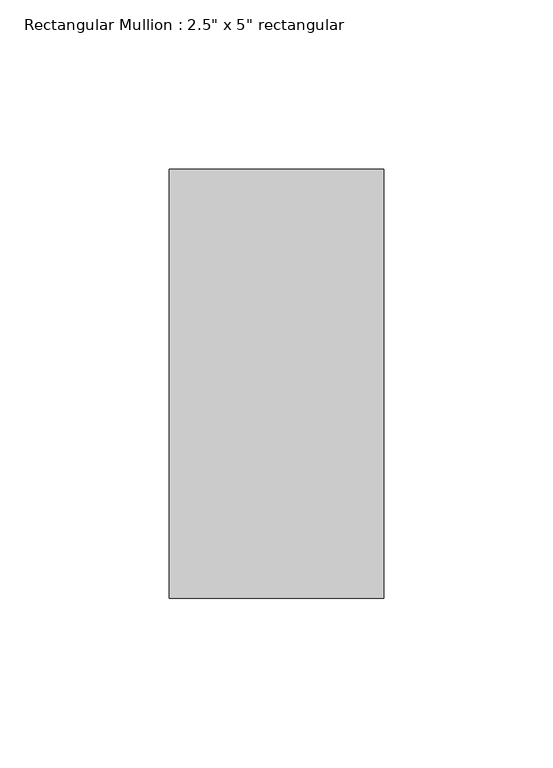
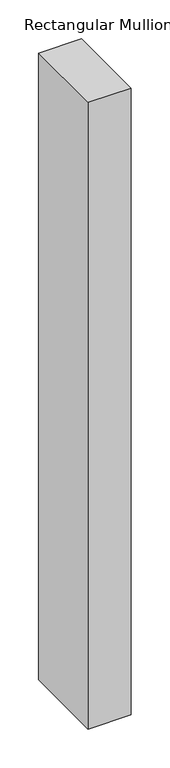
"""IFC4 building model written with IfcOpenShell, lengths in millimetres: member geometry."""

from ifc_helpers import new_model, si_unit, frame, origin, place, context, project, spatial, polyline, outline, extrude, source, transform, mapped, element, save


def member_9fb0cd34(model_context):
    return source(origin(), model_context, "Body", "SweptSolid", [
        extrude(outline(polyline([(31.75, 63.5), (31.75, -63.5), (-31.75, -63.5), (-31.75, 63.5), (31.75, 63.5)])), frame((0.0, 0.0, -983.0943516), z_axis=(0.0, 0.0, 1.0), x_axis=(1.0, 0.0, 0.0)), (0.0, 0.0, 1.0), 983.0943516),
    ])


if __name__ == "__main__":
    model = new_model("IFC4")
    model_context = context("Model", 3, world=origin())
    ifc_project = project(units=[si_unit("LENGTHUNIT", "METRE", prefix="MILLI")], contexts=[model_context])
    site = spatial("IfcSite", under=ifc_project)
    building = spatial("IfcBuilding", under=site)
    placement = place(None, origin())
    member_shape = member_9fb0cd34(model_context)
    element("IfcMember", 1, ObjectType="Rectangular Mullion : 2.5\" x 5\" rectangular", at=placement, inside=building, context=model_context, shape_type="MappedRepresentation", body=[
        mapped(member_shape, transform((0.0, 0.0, 0.0), x_axis=(1.0, 0.0, 0.0), y_axis=(0.0, 1.0, 0.0), z_axis=(0.0, 0.0, 1.0))),
    ])
    save(model, "model.ifc")

# Revit data of these elements
# Type "Rectangular Mullion : 2.5\" x 5\" rectangular"
#   built-in parameter 1007304 = 0.416667 (stored number, unit not read)
#   built-in parameter 1007301 = 0.104167 (stored number, unit not read)
#   built-in parameter 1007300 = 0.104167 (stored number, unit not read)
# Element 1 (IfcMember, "Rectangular Mullion : 2.5\" x 5\" rectangular")
#   Materials on its faces: "Aluminum"
# Materials
#   "Aluminum": class "Metal", colour RGB 247 247 247, transparency 0, Description = "Aluminum 6061", Cost = 0
